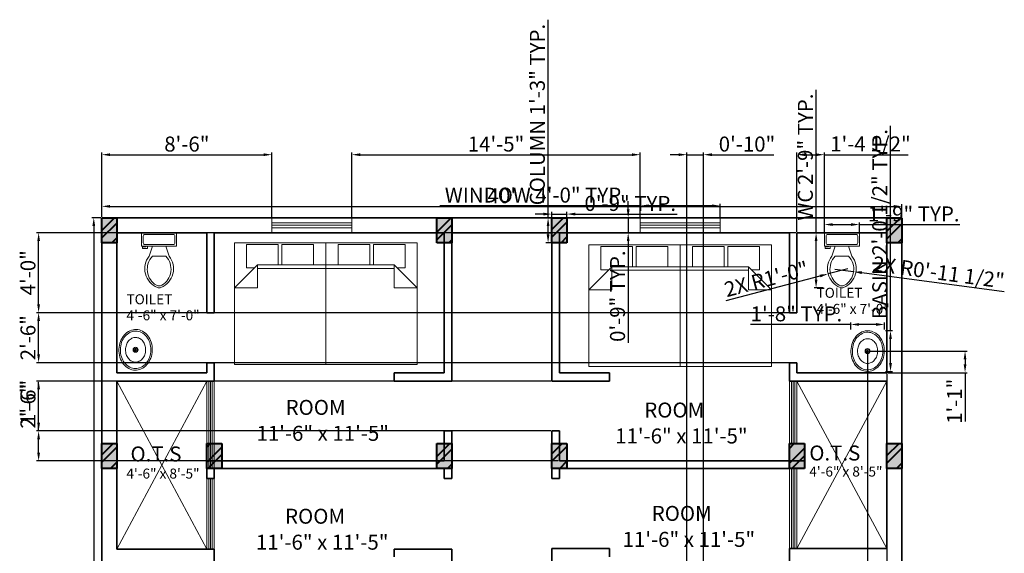
# Model space of a CAD drawing. Units: inches. Extents: x 2507 to 5802, y 1229 to 3238.
# Tile 2 of 2: x 2507 to 3097, y 1794 to 2114. Entities that reach past the tile are written whole.
import ezdxf

# ---------------------------------------------------------------- set-up
doc = ezdxf.new("R2010")
doc.units = ezdxf.units.IN
for name, color, linetype, lineweight, true_color in [('A-ANNO-DIMS', 244, 'Continuous', 18, 0x991b1e), ('A-AREA-IDEN', 146, 'Continuous', 18, 0x105689), ('A-FLOR-FIXT', 244, 'Continuous', 18, 0x991b1e), ('A-FLOR-OPEN', 244, 'Continuous', 13, 0x991b1e), ('A-FURN', 146, 'Continuous', 18, 0x105689), ('A-GLAZ', 146, 'Continuous', 18, 0x105689)]:
    doc.layers.add(name, color=color, linetype=linetype, lineweight=lineweight, true_color=true_color)
doc.layers.add('A-COLS', color=7, linetype='Continuous', lineweight=40)
doc.layers.add('A-WALL', color=7, linetype='Continuous', lineweight=35)
doc.styles.get("Standard").update_dxf_attribs({"font": 'arial.ttf'})
doc.dimstyles.new('ISO-25', dxfattribs={"dimtxt": 9, "dimasz": 5, "dimexe": 1.25, "dimexo": 0.625, "dimtad": 1, "dimdec": 0, "dimlunit": 3, "dimtxsty": 'Standard', "dimcen": 2.5, "dimadec": 0, "dimazin": 0, "dimtfac": 1, "dimtdec": 0, "dimtmove": 0, "dimatfit": 3, "dimfxl": 1, "dimarcsym": 0})
pattern_1 = [(45, (-3102.79, -1462.177), (-6.735192, 6.735192), []), (45, (-3098.3, -1462.177), (-6.735192, 6.735192), [])]

# ---------------------------------------------------------------- blocks, each defined once
blk = doc.blocks.new('Bed - Queen')
for p, q in [((0, -80.00003), (0, 0)), ((0, 0), (59.99999, 0)), ((59.99999, 0), (59.99999, -80.00003)), ((7.99999, -1.2), (28.79998, -1.2)), ((7.99999, -14.4), (7.99999, -1.2)), ((28.79998, -1.2), (28.79998, -14.4)), ((31.19999, -1.2), (51.99999, -1.2)), ((31.19999, -14.4), (31.19999, -1.2)), ((51.99999, -1.2), (51.99999, -16.4)), ((0, -14.4), (44.8, -14.4)), ((44.8, -16.8), (0, -16.8)), ((59.99999, -29.6), (44.8, -14.4)), ((44.8, -14.4), (44.8, -29.6)), ((51.99999, -16.4), (46.79936, -16.4)), ((44.8, -29.6), (59.99999, -29.6)), ((59.99999, -80.00003), (0, -80.00003))]:
    blk.add_line(p, q)
blk = doc.blocks.new('*D2')
at = {"layer": 'A-ANNO-DIMS', "color": 0, "lineweight": -2, "transparency": 16777216}
for p, q in [((2555.99, 1995.72), (2555.99, 2003.23)), ((3035.99, 1995.72), (3035.99, 2003.23)), ((2560.99, 2001.98), (3030.99, 2001.98))]:
    blk.add_line(p, q, dxfattribs=at)
at = {"layer": 'A-ANNO-DIMS', "color": 0, "transparency": 16777216}
for points in [[(2560.99, 2002.81), (2560.99, 2001.15), (2555.99, 2001.98)], [(3030.99, 2002.81), (3030.99, 2001.15), (3035.99, 2001.98)]]:
    blk.add_solid(points, dxfattribs=at)
at = {"layer": 'Defpoints', "color": 0, "transparency": 16777216}
for p in [(3035.99, 2001.98), (2555.99, 1995.09), (3035.99, 1995.09)]:
    blk.add_point(p, dxfattribs=at)
at = {"layer": 'A-ANNO-DIMS', "color": 0, "transparency": 16777216, "insert": (2795.99, 2007.2), "char_height": 9, "attachment_point": 5}
blk.add_mtext("40'", dxfattribs=at)
blk = doc.blocks.new('*D3')
at = {"layer": 'A-ANNO-DIMS', "color": 0, "lineweight": -2, "transparency": 16777216}
for p, q in [((2555.37, 1995.09), (2549.93, 1995.09)), ((2551.18, 1990.09), (2551.18, 1280.09)), ((2555.37, 1275.09), (2549.93, 1275.09))]:
    blk.add_line(p, q, dxfattribs=at)
at = {"layer": 'A-ANNO-DIMS', "color": 0, "transparency": 16777216}
for points in [[(2550.35, 1990.09), (2552.02, 1990.09), (2551.18, 1995.09)], [(2550.35, 1280.09), (2552.02, 1280.09), (2551.18, 1275.09)]]:
    blk.add_solid(points, dxfattribs=at)
at = {"layer": 'Defpoints', "color": 0, "transparency": 16777216}
for p in [(2555.99, 1995.09), (2551.18, 1275.09), (2555.99, 1275.09)]:
    blk.add_point(p, dxfattribs=at)
at = {"layer": 'A-ANNO-DIMS', "color": 0, "transparency": 16777216, "insert": (2545.96, 1635.09), "char_height": 9, "attachment_point": 5, "rotation": 90}
blk.add_mtext("60'", dxfattribs=at)
blk = doc.blocks.new('Toilet - top')
for p, q in [((9.5, -6), (9.5, -2)), ((-10, -8.5), (-8, -8.5)), ((-10, -9.5), (-10, -8.5)), ((-7, -9.5), (-10, -9.5)), ((-8, -8.5), (-8, -8)), ((-7, -8), (-7, -9.5)), ((-4, -8), (-6, -14)), ((4, -8), (6, -14)), ((4, -14), (-4, -14))]:
    blk.add_line(p, q)
blk.add_lwpolyline([(10.5, -8), (10.5, 0), (-10.5, 0), (-10.5, -8)], close=True)
for points in [[(-9.5, -2), (-9.5, -6)], [(8.5, -1), (-8.5, -1)], [(-8.5, -7), (8.5, -7)]]:
    blk.add_lwpolyline(points)
for centre, radius, start, end in [((-8.62, -1.88), 0.884, 81.8699, 188.1301), ((8.62, -1.88), 0.884, 351.8699, 98.1301), ((-8.62, -6.12), 0.884, 171.8699, 278.1301), ((8.62, -6.12), 0.884, 261.8699, 8.1301), ((3.52, -21.58), 12.17, 141.46911, 247.97143), ((4.2, -21.82), 11.33, 136.36773, 238.94682), ((-3.52, -21.58), 12.17, 292.02843, 38.53071), ((-4.2, -21.82), 11.33, 301.05301, 43.63209), ((0, -27.88), 4, 245.73182, 294.26817), ((0, -29), 4, 254.86053, 285.13947)]:
    blk.add_arc(centre, radius, start, end)
blk = doc.blocks.new('Sink - Oval top')
for p, q in [((-1, 0), (1, 0)), ((0, 1), (0, -1))]:
    blk.add_line(p, q)
for points in [[(-12.23, 0.39, 0.117634), (-11.46, -3.36, 0.104469), (-8.88, -6.8, 0.090016), (-5.08, -9.07, 0.08192), (-0.32, -10.02, 0.08192), (4.49, -9.38, 0.090016), (8.42, -7.36, 0.104469), (11.22, -4.09, 0.117634), (12.23, -0.39, 0.117634), (11.46, 3.36, 0.104469), (8.88, 6.8, 0.090016), (5.08, 9.07, 0.08192), (0.32, 10.02, 0.08192), (-4.49, 9.38, 0.090016), (-8.42, 7.36, 0.104469), (-11.22, 4.09, 0.117634)], [(-11.29, 0.16, 0.118622), (-10.52, -3.25, 0.104678), (-8.07, -6.36, 0.089562), (-4.54, -8.37, 0.081185), (-0.13, -9.15, 0.081185), (4.3, -8.49, 0.089562), (7.89, -6.58, 0.104678), (10.42, -3.55, 0.118622), (11.29, -0.16, 0.118622), (10.52, 3.25, 0.104678), (8.07, 6.36, 0.089562), (4.54, 8.37, 0.081185), (0.13, 9.15, 0.081185), (-4.3, 8.49, 0.089562), (-7.89, 6.58, 0.104678), (-10.42, 3.55, 0.118622)], [(-7.42, 0.08, 0.118283), (-6.91, -2.17, 0.104607), (-5.29, -4.21, 0.089718), (-2.97, -5.53, 0.081436), (-0.07, -6.04, 0.081436), (2.84, -5.59, 0.089718), (5.2, -4.33, 0.104607), (6.86, -2.32, 0.118283), (7.42, -0.08, 0.118283), (6.91, 2.17, 0.104607), (5.29, 4.21, 0.089718), (2.97, 5.53, 0.081436), (0.07, 6.04, 0.081436), (-2.84, 5.59, 0.089718), (-5.2, 4.33, 0.104607), (-6.86, 2.32, 0.118283)]]:
    blk.add_lwpolyline(points, format="xyb", close=True)
for radius in [1.5, 1]:
    blk.add_circle((0, 0), radius)
blk = doc.blocks.new('COL-9x15')
h = blk.add_hatch()
h.set_pattern_fill('ANSI32', color=256)
h.set_pattern_definition(pattern_1)
h.paths.add_polyline_path([(9, 15), (0, 15), (0, 0), (9, 0)])
h = blk.add_hatch()
h.set_pattern_fill('ANSI32', color=256)
h.set_pattern_definition(pattern_1)
h.paths.add_polyline_path([(9, 15), (0, 15), (0, 0), (9, 0)])
at = {"transparency": 33554687}
h = blk.add_hatch(dxfattribs=at)
h.set_pattern_fill('ANSI32', color=256)
h.set_pattern_definition(pattern_1)
h.paths.add_polyline_path([(9, 15), (0, 15), (0, 0), (9, 0)])
h = blk.add_hatch(color=256, dxfattribs=at)
h.dxf.hatch_style = 1
h.paths.add_polyline_path([(9, 15), (0, 15), (0, 0), (9, 0)])
for p, q in [((0, 15), (9, 15)), ((0, 0), (0, 15)), ((9, 15), (9, 0)), ((9, 0), (0, 0))]:
    blk.add_line(p, q)
blk = doc.blocks.new('WIN-48x9')
for p, q in [((0, 9), (48, 9)), ((0, 0), (0, 9)), ((0, 6), (48, 6)), ((48, 9), (48, 0)), ((0, 4.5), (48, 4.5)), ((0, 3), (48, 3)), ((48, 0), (0, 0))]:
    blk.add_line(p, q)
blk = doc.blocks.new('*D13')
at = {"layer": 'A-ANNO-DIMS', "color": 0, "lineweight": -2, "transparency": 16777216}
for p, q in [((2823.74, 1995.09), (2823.74, 2114.07)), ((2825.37, 1995.09), (2822.49, 1995.09)), ((2823.74, 1985.09), (2823.74, 1990.09)), ((2825.37, 1980.09), (2822.49, 1980.09))]:
    blk.add_line(p, q, dxfattribs=at)
at = {"layer": 'A-ANNO-DIMS', "color": 0, "transparency": 16777216}
for points in [[(2822.91, 1990.09), (2824.57, 1990.09), (2823.74, 1995.09)], [(2822.91, 1985.09), (2824.57, 1985.09), (2823.74, 1980.09)]]:
    blk.add_solid(points, dxfattribs=at)
at = {"layer": 'Defpoints', "color": 0, "transparency": 16777216}
for p in [(2823.74, 1995.09), (2825.99, 1995.09), (2825.99, 1980.09)]:
    blk.add_point(p, dxfattribs=at)
at = {"layer": 'A-ANNO-DIMS', "color": 0, "transparency": 16777216, "insert": (2818.46, 2057.08), "char_height": 9, "attachment_point": 5, "rotation": 90}
blk.add_mtext('COLUMN 1\'-3" TYP.', dxfattribs=at)
blk = doc.blocks.new('*D14')
at = {"layer": 'A-ANNO-DIMS', "color": 0, "lineweight": -2, "transparency": 16777216}
for p, q in [((2820.99, 1997.34), (2815.99, 1997.34)), ((2825.99, 1995.72), (2825.99, 1998.59)), ((2825.99, 1997.34), (2834.99, 1997.34)), ((2834.99, 1995.72), (2834.99, 1998.59)), ((2839.99, 1997.34), (2901.1, 1997.34))]:
    blk.add_line(p, q, dxfattribs=at)
at = {"layer": 'A-ANNO-DIMS', "color": 0, "transparency": 16777216}
for points in [[(2820.99, 1998.17), (2820.99, 1996.51), (2825.99, 1997.34)], [(2839.99, 1998.17), (2839.99, 1996.51), (2834.99, 1997.34)]]:
    blk.add_solid(points, dxfattribs=at)
at = {"layer": 'Defpoints', "color": 0, "transparency": 16777216}
for p in [(2834.99, 1997.34), (2825.99, 1995.09), (2834.99, 1995.09)]:
    blk.add_point(p, dxfattribs=at)
at = {"layer": 'A-ANNO-DIMS', "color": 0, "transparency": 16777216, "insert": (2873.04, 2002.56), "char_height": 9, "attachment_point": 5}
blk.add_mtext('0\'-9" TYP.', dxfattribs=at)
blk = doc.blocks.new('*D17')
at = {"layer": 'A-ANNO-DIMS', "color": 0, "lineweight": -2, "transparency": 16777216}
for p, q in [((2984.53, 1986.09), (2984.53, 2072.01)), ((2988.87, 1986.09), (2983.28, 1986.09)), ((2984.53, 1958.04), (2984.53, 1981.09)), ((2988.87, 1953.04), (2983.28, 1953.04))]:
    blk.add_line(p, q, dxfattribs=at)
at = {"layer": 'A-ANNO-DIMS', "color": 0, "transparency": 16777216}
for points in [[(2983.7, 1981.09), (2985.37, 1981.09), (2984.53, 1986.09)], [(2983.7, 1958.04), (2985.37, 1958.04), (2984.53, 1953.04)]]:
    blk.add_solid(points, dxfattribs=at)
at = {"layer": 'Defpoints', "color": 0, "transparency": 16777216}
for p in [(2984.53, 1986.09), (2989.49, 1986.09), (2989.49, 1953.04)]:
    blk.add_point(p, dxfattribs=at)
at = {"layer": 'A-ANNO-DIMS', "color": 0, "transparency": 16777216, "insert": (2979.25, 2031.55), "char_height": 9, "attachment_point": 5, "rotation": 90}
blk.add_mtext('WC 2\'-9" TYP.', dxfattribs=at)
blk = doc.blocks.new('*D18')
at = {"layer": 'A-ANNO-DIMS', "color": 0, "lineweight": -2, "transparency": 16777216}
for p, q in [((2989.49, 1986.72), (2989.49, 1992.3)), ((2994.49, 1991.05), (3005.49, 1991.05)), ((3010.49, 1986.72), (3010.49, 1992.3)), ((3010.49, 1991.05), (3070.75, 1991.05))]:
    blk.add_line(p, q, dxfattribs=at)
at = {"layer": 'A-ANNO-DIMS', "color": 0, "transparency": 16777216}
for points in [[(2994.49, 1991.88), (2994.49, 1990.21), (2989.49, 1991.05)], [(3005.49, 1991.88), (3005.49, 1990.21), (3010.49, 1991.05)]]:
    blk.add_solid(points, dxfattribs=at)
at = {"layer": 'Defpoints', "color": 0, "transparency": 16777216}
for p in [(3010.49, 1991.05), (2989.49, 1986.09), (3010.49, 1986.09)]:
    blk.add_point(p, dxfattribs=at)
at = {"layer": 'A-ANNO-DIMS', "color": 0, "transparency": 16777216, "insert": (3043.12, 1996.27), "char_height": 9, "attachment_point": 5}
blk.add_mtext('1\'-9" TYP.', dxfattribs=at)
blk = doc.blocks.new('*D19')
at = {"layer": 'A-ANNO-DIMS', "color": 0, "lineweight": -2, "transparency": 16777216}
for p, q in [((3029.18, 1927.36), (3029.18, 2050.27)), ((3026.12, 1927.36), (3030.43, 1927.36)), ((3029.18, 1907.81), (3029.18, 1922.36)), ((3026.12, 1902.81), (3030.43, 1902.81))]:
    blk.add_line(p, q, dxfattribs=at)
at = {"layer": 'A-ANNO-DIMS', "color": 0, "transparency": 16777216}
for points in [[(3028.34, 1922.36), (3030.01, 1922.36), (3029.18, 1927.36)], [(3028.34, 1907.81), (3030.01, 1907.81), (3029.18, 1902.81)]]:
    blk.add_solid(points, dxfattribs=at)
at = {"layer": 'Defpoints', "color": 0, "transparency": 16777216}
for p in [(3025.49, 1927.36), (3029.18, 1927.36), (3025.49, 1902.81)]:
    blk.add_point(p, dxfattribs=at)
at = {"layer": 'A-ANNO-DIMS', "color": 0, "transparency": 16777216, "insert": (3023.9, 1991.31), "char_height": 9, "attachment_point": 5, "rotation": 90}
blk.add_mtext('BASIN 2\'-0 1/2" TYP.', dxfattribs=at)
blk = doc.blocks.new('*D20')
at = {"layer": 'A-ANNO-DIMS', "color": 0, "lineweight": -2, "transparency": 16777216}
for p, q in [((3005.36, 1927.98), (3005.36, 1932.29)), ((3025.49, 1927.98), (3025.49, 1932.29)), ((3005.36, 1931.04), (2945.1, 1931.04)), ((3020.49, 1931.04), (3010.36, 1931.04))]:
    blk.add_line(p, q, dxfattribs=at)
at = {"layer": 'A-ANNO-DIMS', "color": 0, "transparency": 16777216}
for points in [[(3010.36, 1931.88), (3010.36, 1930.21), (3005.36, 1931.04)], [(3020.49, 1931.88), (3020.49, 1930.21), (3025.49, 1931.04)]]:
    blk.add_solid(points, dxfattribs=at)
at = {"layer": 'Defpoints', "color": 0, "transparency": 16777216}
for p in [(3005.36, 1931.04), (3005.36, 1927.36), (3025.49, 1927.36)]:
    blk.add_point(p, dxfattribs=at)
at = {"layer": 'A-ANNO-DIMS', "color": 0, "transparency": 16777216, "insert": (2972.73, 1936.26), "char_height": 9, "attachment_point": 5}
blk.add_mtext('1\'-8" TYP.', dxfattribs=at)
blk = doc.blocks.new('*D21')
at = {"layer": 'A-ANNO-DIMS', "color": 0, "lineweight": -2, "transparency": 16777216}
for p, q in [((2878.99, 1995.72), (2878.99, 2003.54)), ((2926.99, 1995.72), (2926.99, 2003.54)), ((2878.99, 2002.29), (2758.86, 2002.29)), ((2921.99, 2002.29), (2883.99, 2002.29))]:
    blk.add_line(p, q, dxfattribs=at)
at = {"layer": 'A-ANNO-DIMS', "color": 0, "transparency": 16777216}
for points in [[(2883.99, 2003.12), (2883.99, 2001.46), (2878.99, 2002.29)], [(2921.99, 2003.12), (2921.99, 2001.46), (2926.99, 2002.29)]]:
    blk.add_solid(points, dxfattribs=at)
at = {"layer": 'Defpoints', "color": 0, "transparency": 16777216}
for p in [(2878.99, 2002.29), (2878.99, 1995.09), (2926.99, 1995.09)]:
    blk.add_point(p, dxfattribs=at)
at = {"layer": 'A-ANNO-DIMS', "color": 0, "transparency": 16777216, "insert": (2816.42, 2007.57), "char_height": 9, "attachment_point": 5}
blk.add_mtext('WINDOW 4\'-0" TYP.', dxfattribs=at)
blk = doc.blocks.new('*D22')
at = {"layer": 'A-ANNO-DIMS', "color": 0, "lineweight": -2, "transparency": 16777216}
for p, q in [((2871.79, 2000.09), (2871.79, 2005.09)), ((2878.37, 1995.09), (2870.54, 1995.09)), ((2871.79, 1995.09), (2871.79, 1986.09)), ((2878.37, 1986.09), (2870.54, 1986.09)), ((2871.79, 1981.09), (2871.79, 1919.98))]:
    blk.add_line(p, q, dxfattribs=at)
at = {"layer": 'A-ANNO-DIMS', "color": 0, "transparency": 16777216}
for points in [[(2870.96, 2000.09), (2872.63, 2000.09), (2871.79, 1995.09)], [(2870.96, 1981.09), (2872.63, 1981.09), (2871.79, 1986.09)]]:
    blk.add_solid(points, dxfattribs=at)
at = {"layer": 'Defpoints', "color": 0, "transparency": 16777216}
for p in [(2878.99, 1995.09), (2871.79, 1986.09), (2878.99, 1986.09)]:
    blk.add_point(p, dxfattribs=at)
at = {"layer": 'A-ANNO-DIMS', "color": 0, "transparency": 16777216, "insert": (2866.57, 1948.04), "char_height": 9, "attachment_point": 5, "rotation": 90}
blk.add_mtext('0\'-9" TYP.', dxfattribs=at)
blk = doc.blocks.new('*D25')
at = {"layer": 'A-ANNO-DIMS', "color": 0, "lineweight": -2, "transparency": 16777216}
for p, q in [((2555.99, 1995.72), (2555.99, 2034.24)), ((2560.99, 2032.99), (2653.02, 2032.99)), ((2658.02, 1995.72), (2658.02, 2034.24))]:
    blk.add_line(p, q, dxfattribs=at)
at = {"layer": 'A-ANNO-DIMS', "color": 0, "transparency": 16777216}
for points in [[(2560.99, 2033.82), (2560.99, 2032.16), (2555.99, 2032.99)], [(2653.02, 2033.82), (2653.02, 2032.16), (2658.02, 2032.99)]]:
    blk.add_solid(points, dxfattribs=at)
at = {"layer": 'Defpoints', "color": 0, "transparency": 16777216}
for p in [(2658.02, 2032.99), (2555.99, 1995.09), (2658.02, 1995.09)]:
    blk.add_point(p, dxfattribs=at)
at = {"layer": 'A-ANNO-DIMS', "color": 0, "transparency": 16777216, "insert": (2607.01, 2038.21), "char_height": 9, "attachment_point": 5}
blk.add_mtext('8\'-6"', dxfattribs=at)
blk = doc.blocks.new('*D26')
at = {"layer": 'A-ANNO-DIMS', "color": 0, "lineweight": -2, "transparency": 16777216}
for p, q in [((2706.02, 1995.72), (2706.02, 2034.24)), ((2711.02, 2032.99), (2873.99, 2032.99)), ((2878.99, 1995.72), (2878.99, 2034.24))]:
    blk.add_line(p, q, dxfattribs=at)
at = {"layer": 'A-ANNO-DIMS', "color": 0, "transparency": 16777216}
for points in [[(2711.02, 2033.82), (2711.02, 2032.16), (2706.02, 2032.99)], [(2873.99, 2033.82), (2873.99, 2032.16), (2878.99, 2032.99)]]:
    blk.add_solid(points, dxfattribs=at)
at = {"layer": 'Defpoints', "color": 0, "transparency": 16777216}
for p in [(2878.99, 2032.99), (2706.02, 1995.09), (2878.99, 1995.09)]:
    blk.add_point(p, dxfattribs=at)
at = {"layer": 'A-ANNO-DIMS', "color": 0, "transparency": 16777216, "insert": (2792.51, 2038.21), "char_height": 9, "attachment_point": 5}
blk.add_mtext('14\'-5"', dxfattribs=at)
blk = doc.blocks.new('*D30')
at = {"layer": 'A-ANNO-DIMS', "color": 0, "lineweight": -2, "transparency": 16777216}
for p, q in [((2825.37, 1897.09), (2516.84, 1897.09)), ((2518.09, 1872.09), (2518.09, 1892.09)), ((2825.37, 1867.09), (2516.84, 1867.09))]:
    blk.add_line(p, q, dxfattribs=at)
at = {"layer": 'A-ANNO-DIMS', "color": 0, "transparency": 16777216}
for points in [[(2517.26, 1892.09), (2518.92, 1892.09), (2518.09, 1897.09)], [(2517.26, 1872.09), (2518.92, 1872.09), (2518.09, 1867.09)]]:
    blk.add_solid(points, dxfattribs=at)
at = {"layer": 'Defpoints', "color": 0, "transparency": 16777216}
for p in [(2518.09, 1897.09), (2825.99, 1897.09), (2825.99, 1867.09)]:
    blk.add_point(p, dxfattribs=at)
at = {"layer": 'A-ANNO-DIMS', "color": 0, "transparency": 16777216, "insert": (2512.87, 1882.09), "char_height": 9, "attachment_point": 5, "rotation": 90}
blk.add_mtext('2\'-6"', dxfattribs=at)
blk = doc.blocks.new('*D31')
at = {"layer": 'A-ANNO-DIMS', "color": 0, "lineweight": -2, "transparency": 16777216}
for p, q in [((2518.09, 1867.09), (2518.09, 1896.42)), ((2825.37, 1867.09), (2516.84, 1867.09)), ((2518.09, 1854.09), (2518.09, 1862.09)), ((2829.87, 1849.09), (2516.84, 1849.09))]:
    blk.add_line(p, q, dxfattribs=at)
at = {"layer": 'A-ANNO-DIMS', "color": 0, "transparency": 16777216}
for points in [[(2517.26, 1862.09), (2518.92, 1862.09), (2518.09, 1867.09)], [(2517.26, 1854.09), (2518.92, 1854.09), (2518.09, 1849.09)]]:
    blk.add_solid(points, dxfattribs=at)
at = {"layer": 'Defpoints', "color": 0, "transparency": 16777216}
for p in [(2518.09, 1867.09), (2825.99, 1867.09), (2830.49, 1849.09)]:
    blk.add_point(p, dxfattribs=at)
at = {"layer": 'A-ANNO-DIMS', "color": 0, "transparency": 16777216, "insert": (2512.87, 1884.25), "char_height": 9, "attachment_point": 5, "rotation": 90}
blk.add_mtext('1\'-6"', dxfattribs=at)
blk = doc.blocks.new('*D32')
at = {"layer": 'A-ANNO-DIMS', "color": 0, "lineweight": -2, "transparency": 16777216}
for p, q in [((2972.37, 1938.09), (2516.84, 1938.09)), ((2518.09, 1913.09), (2518.09, 1933.09)), ((2972.37, 1908.09), (2516.84, 1908.09))]:
    blk.add_line(p, q, dxfattribs=at)
at = {"layer": 'A-ANNO-DIMS', "color": 0, "transparency": 16777216}
for points in [[(2517.26, 1933.09), (2518.92, 1933.09), (2518.09, 1938.09)], [(2517.26, 1913.09), (2518.92, 1913.09), (2518.09, 1908.09)]]:
    blk.add_solid(points, dxfattribs=at)
at = {"layer": 'Defpoints', "color": 0, "transparency": 16777216}
for p in [(2518.09, 1938.09), (2972.99, 1938.09), (2972.99, 1908.09)]:
    blk.add_point(p, dxfattribs=at)
at = {"layer": 'A-ANNO-DIMS', "color": 0, "transparency": 16777216, "insert": (2512.87, 1923.09), "char_height": 9, "attachment_point": 5, "rotation": 90}
blk.add_mtext('2\'-6"', dxfattribs=at)
blk = doc.blocks.new('*D33')
at = {"layer": 'A-ANNO-DIMS', "color": 0, "lineweight": -2, "transparency": 16777216}
for p, q in [((2972.37, 1986.09), (2516.84, 1986.09)), ((2518.09, 1943.09), (2518.09, 1981.09)), ((2972.37, 1938.09), (2516.84, 1938.09))]:
    blk.add_line(p, q, dxfattribs=at)
at = {"layer": 'A-ANNO-DIMS', "color": 0, "transparency": 16777216}
for points in [[(2517.26, 1981.09), (2518.92, 1981.09), (2518.09, 1986.09)], [(2517.26, 1943.09), (2518.92, 1943.09), (2518.09, 1938.09)]]:
    blk.add_solid(points, dxfattribs=at)
at = {"layer": 'Defpoints', "color": 0, "transparency": 16777216}
for p in [(2518.09, 1986.09), (2972.99, 1986.09), (2972.99, 1938.09)]:
    blk.add_point(p, dxfattribs=at)
at = {"layer": 'A-ANNO-DIMS', "color": 0, "transparency": 16777216, "insert": (2512.87, 1962.09), "char_height": 9, "attachment_point": 5, "rotation": 90}
blk.add_mtext('4\'-0"', dxfattribs=at)
blk = doc.blocks.new('*D34')
at = {"layer": 'A-ANNO-DIMS', "color": 0, "lineweight": -2, "transparency": 16777216}
for p, q in [((2901.99, 2032.99), (2896.99, 2032.99)), ((2906.99, 1344.72), (2906.99, 2034.24)), ((2906.99, 2032.99), (2916.99, 2032.99)), ((2916.99, 1344.72), (2916.99, 2034.24)), ((2921.99, 2032.99), (2959.16, 2032.99))]:
    blk.add_line(p, q, dxfattribs=at)
at = {"layer": 'A-ANNO-DIMS', "color": 0, "transparency": 16777216}
for points in [[(2901.99, 2033.82), (2901.99, 2032.16), (2906.99, 2032.99)], [(2921.99, 2033.82), (2921.99, 2032.16), (2916.99, 2032.99)]]:
    blk.add_solid(points, dxfattribs=at)
at = {"layer": 'Defpoints', "color": 0, "transparency": 16777216}
for p in [(2916.99, 2032.99), (2906.99, 1344.09), (2916.99, 1344.09)]:
    blk.add_point(p, dxfattribs=at)
at = {"layer": 'A-ANNO-DIMS', "color": 0, "transparency": 16777216, "insert": (2943.07, 2038.21), "char_height": 9, "attachment_point": 5}
blk.add_mtext('0\'-10"', dxfattribs=at)
blk = doc.blocks.new('*D36')
at = {"layer": 'A-ANNO-DIMS', "color": 0, "lineweight": -2, "transparency": 16777216}
for p, q in [((2972.99, 1986.72), (2972.99, 2034.24)), ((2977.99, 2032.99), (2984.49, 2032.99)), ((2989.49, 1986.72), (2989.49, 2034.24)), ((2989.49, 2032.99), (3039.79, 2032.99))]:
    blk.add_line(p, q, dxfattribs=at)
at = {"layer": 'A-ANNO-DIMS', "color": 0, "transparency": 16777216}
for points in [[(2977.99, 2033.82), (2977.99, 2032.16), (2972.99, 2032.99)], [(2984.49, 2033.82), (2984.49, 2032.16), (2989.49, 2032.99)]]:
    blk.add_solid(points, dxfattribs=at)
at = {"layer": 'Defpoints', "color": 0, "transparency": 16777216}
for p in [(2989.49, 2032.99), (2972.99, 1986.09), (2989.49, 1986.09)]:
    blk.add_point(p, dxfattribs=at)
at = {"layer": 'A-ANNO-DIMS', "color": 0, "transparency": 16777216, "insert": (3017.14, 2038.27), "char_height": 9, "attachment_point": 5}
blk.add_mtext('1\'-4 1/2"', dxfattribs=at)
blk = doc.blocks.new('*D37')
at = {"layer": 'A-ANNO-DIMS', "color": 0, "lineweight": -2, "transparency": 16777216}
for p, q in [((3015.43, 1914.46), (3015.43, 1235.94)), ((3026.99, 1901.47), (3026.99, 1235.94)), ((3020.43, 1237.19), (3021.99, 1237.19)), ((3026.99, 1237.19), (3085.13, 1237.19))]:
    blk.add_line(p, q, dxfattribs=at)
at = {"layer": 'A-ANNO-DIMS', "color": 0, "transparency": 16777216}
for points in [[(3020.43, 1238.02), (3020.43, 1236.36), (3015.43, 1237.19)], [(3021.99, 1238.02), (3021.99, 1236.36), (3026.99, 1237.19)]]:
    blk.add_solid(points, dxfattribs=at)
at = {"layer": 'Defpoints', "color": 0, "transparency": 16777216}
for p in [(3015.43, 1915.08), (3026.99, 1902.09), (3026.99, 1237.19)]:
    blk.add_point(p, dxfattribs=at)
at = {"layer": 'A-ANNO-DIMS', "color": 0, "transparency": 16777216, "insert": (3058.56, 1242.47), "char_height": 9, "attachment_point": 5}
blk.add_mtext('0\'-11 1/2"', dxfattribs=at)
blk = doc.blocks.new('*D38')
at = {"layer": 'A-ANNO-DIMS', "color": 0, "lineweight": -2, "transparency": 16777216}
for p, q in [((3016.05, 1915.08), (3075.14, 1915.08)), ((3073.89, 1910.08), (3073.89, 1907.09)), ((3027.62, 1902.09), (3075.14, 1902.09)), ((3073.89, 1902.09), (3073.89, 1872.76))]:
    blk.add_line(p, q, dxfattribs=at)
at = {"layer": 'A-ANNO-DIMS', "color": 0, "transparency": 16777216}
for points in [[(3073.06, 1910.08), (3074.72, 1910.08), (3073.89, 1915.08)], [(3073.06, 1907.09), (3074.72, 1907.09), (3073.89, 1902.09)]]:
    blk.add_solid(points, dxfattribs=at)
at = {"layer": 'Defpoints', "color": 0, "transparency": 16777216}
for p in [(3015.43, 1915.08), (3026.99, 1902.09), (3073.89, 1902.09)]:
    blk.add_point(p, dxfattribs=at)
at = {"layer": 'A-ANNO-DIMS', "color": 0, "transparency": 16777216, "insert": (3068.75, 1884.93), "char_height": 9, "attachment_point": 5, "rotation": 90}
blk.add_mtext('1\'-1"', dxfattribs=at)
blk = doc.blocks.new('*D39')
at = {"layer": 'A-ANNO-DIMS', "color": 0, "lineweight": -2, "transparency": 16777216}
for p, q in [((3003.51, 1964.51), (2991.74, 1961.42)), ((2930.54, 1945.34), (2986.9, 1960.15))]:
    blk.add_line(p, q, dxfattribs=at)
at = {"layer": 'A-ANNO-DIMS', "color": 0, "transparency": 16777216}
blk.add_solid([(2986.69, 1960.95), (2987.12, 1959.34), (2991.74, 1961.42)], dxfattribs=at)
at = {"layer": 'Defpoints', "color": 0, "transparency": 16777216}
for p in [(2991.74, 1961.42), (3003.51, 1964.51)]:
    blk.add_point(p, dxfattribs=at)
at = {"layer": 'A-ANNO-DIMS', "color": 0, "transparency": 16777216, "insert": (2954.98, 1957.16), "char_height": 9, "attachment_point": 5, "rotation": 14.72153}
blk.add_mtext('2X R1\'-0"', dxfattribs=at)
blk = doc.blocks.new('*D40')
at = {"layer": 'A-ANNO-DIMS', "color": 0, "lineweight": -2, "transparency": 16777216}
for p, q in [((2995.79, 1964.27), (3007.02, 1962.76)), ((3097.45, 1950.61), (3011.97, 1962.1))]:
    blk.add_line(p, q, dxfattribs=at)
at = {"layer": 'A-ANNO-DIMS', "color": 0, "transparency": 16777216}
blk.add_solid([(3012.08, 1962.92), (3011.86, 1961.27), (3007.02, 1962.76)], dxfattribs=at)
at = {"layer": 'Defpoints', "color": 0, "transparency": 16777216}
for p in [(2995.79, 1964.27), (3007.02, 1962.76)]:
    blk.add_point(p, dxfattribs=at)
at = {"layer": 'A-ANNO-DIMS', "color": 0, "transparency": 16777216, "insert": (3057.89, 1961.25), "char_height": 9, "attachment_point": 5, "rotation": 352.34378}
blk.add_mtext('2X R0\'-11 1/2"', dxfattribs=at)

msp = doc.modelspace()

# ---------------------------------------------------------------- linework, layer by layer
at = {"layer": 'A-FLOR-OPEN'}
for p, q in [((2564.99, 1897.09), (2618.99, 1796.09)), ((2564.99, 1796.09), (2618.99, 1897.09)), ((2972.99, 1897.09), (3026.99, 1796.59)), ((2972.99, 1796.59), (3026.99, 1897.09))]:
    msp.add_line(p, q, dxfattribs=at)
at = {"layer": 'A-GLAZ'}
for p, q in [((2618.99, 1897.09), (2618.99, 1844.59)), ((2618.99, 1897.09), (2623.49, 1897.09)), ((2620.24, 1897.09), (2620.24, 1844.59)), ((2621.24, 1897.09), (2621.24, 1844.59)), ((2622.24, 1897.09), (2622.24, 1844.59)), ((2623.49, 1897.09), (2623.49, 1844.59)), ((2968.49, 1897.09), (2972.99, 1897.09)), ((2968.49, 1897.09), (2968.49, 1859.59)), ((2969.74, 1897.09), (2969.74, 1859.59)), ((2970.74, 1897.09), (2970.74, 1859.59)), ((2971.74, 1897.09), (2971.74, 1859.59)), ((2972.99, 1897.09), (2972.99, 1859.59)), ((2968.49, 1796.59), (2968.49, 1844.59)), ((2969.74, 1796.59), (2969.74, 1844.59)), ((2970.74, 1796.59), (2970.74, 1844.59)), ((2971.74, 1796.59), (2971.74, 1844.59)), ((2972.99, 1796.59), (2972.99, 1844.59)), ((2618.99, 1838.59), (2618.99, 1796.09)), ((2620.24, 1838.59), (2620.24, 1796.09)), ((2621.24, 1838.59), (2621.24, 1796.09)), ((2622.24, 1838.59), (2622.24, 1796.09)), ((2623.49, 1838.59), (2623.49, 1796.09)), ((2968.49, 1796.59), (2972.99, 1796.59))]:
    msp.add_line(p, q, dxfattribs=at)
at = {"layer": 'A-WALL'}
for p, q in [((2555.99, 1995.09), (3035.99, 1995.09)), ((2555.99, 1275.09), (2555.99, 1995.09)), ((3035.99, 1995.09), (3035.99, 1275.09)), ((2564.99, 1986.09), (2618.99, 1986.09)), ((2564.99, 1902.09), (2564.99, 1986.09)), ((2618.99, 1938.09), (2618.99, 1986.09)), ((2623.49, 1938.09), (2623.49, 1986.09)), ((2623.49, 1986.09), (2761.49, 1986.09)), ((2761.49, 1902.09), (2761.49, 1986.09)), ((2765.99, 1897.09), (2765.99, 1986.09)), ((2765.99, 1986.09), (2825.99, 1986.09)), ((2825.99, 1908.09), (2825.99, 1986.09)), ((2830.49, 1908.09), (2830.49, 1986.09)), ((2830.49, 1986.09), (2968.49, 1986.09)), ((2968.49, 1938.09), (2968.49, 1986.09)), ((2972.99, 1938.09), (2972.99, 1986.09)), ((2972.99, 1986.09), (3026.99, 1986.09)), ((3026.99, 1986.09), (3026.99, 1902.09)), ((2618.99, 1938.09), (2623.49, 1938.09)), ((2968.49, 1938.09), (2972.99, 1938.09)), ((2618.99, 1902.09), (2618.99, 1908.09)), ((2618.99, 1908.09), (2623.49, 1908.09)), ((2618.99, 1908.09), (2623.49, 1908.09)), ((2623.49, 1897.09), (2623.49, 1908.09)), ((2825.99, 1897.09), (2825.99, 1908.09)), ((2830.49, 1902.09), (2830.49, 1908.09)), ((2968.49, 1908.09), (2972.99, 1908.09)), ((2968.49, 1897.09), (2968.49, 1908.09)), ((2972.99, 1902.09), (2972.99, 1908.09)), ((2564.99, 1902.09), (2618.99, 1902.09)), ((2564.99, 1902.09), (2618.99, 1902.09)), ((2731.49, 1897.09), (2731.49, 1902.09)), ((2731.49, 1902.09), (2761.49, 1902.09)), ((2731.49, 1902.09), (2761.49, 1902.09)), ((2830.49, 1902.09), (2860.49, 1902.09)), ((2860.49, 1897.09), (2860.49, 1902.09)), ((2972.99, 1902.09), (3026.99, 1902.09)), ((2564.99, 1897.09), (2623.49, 1897.09)), ((2564.99, 1897.09), (2623.49, 1897.09)), ((2564.99, 1796.09), (2564.99, 1897.09)), ((2731.49, 1897.09), (2765.99, 1897.09)), ((2731.49, 1897.09), (2765.99, 1897.09)), ((2825.99, 1897.09), (2860.49, 1897.09)), ((2968.49, 1897.09), (3026.99, 1897.09)), ((3026.99, 1897.09), (3026.99, 1849.09)), ((2761.49, 1867.09), (2765.99, 1867.09)), ((2761.49, 1849.09), (2761.49, 1867.09)), ((2765.99, 1838.59), (2765.99, 1867.09)), ((2825.99, 1867.09), (2830.49, 1867.09)), ((2825.99, 1838.59), (2825.99, 1867.09)), ((2830.49, 1849.09), (2830.49, 1867.09)), ((2618.99, 1849.09), (2761.49, 1849.09)), ((2618.99, 1844.59), (2618.99, 1849.09)), ((2830.49, 1849.09), (2977.49, 1849.09)), ((2618.99, 1838.59), (2618.99, 1844.59)), ((2623.49, 1844.59), (2761.49, 1844.59)), ((2623.49, 1838.59), (2623.49, 1844.59)), ((2761.49, 1838.59), (2761.49, 1844.59)), ((2830.49, 1844.59), (2977.49, 1844.59)), ((2830.49, 1838.59), (2830.49, 1844.59)), ((3026.99, 1844.59), (3026.99, 1796.59)), ((2618.99, 1838.59), (2623.49, 1838.59)), ((2761.49, 1838.59), (2765.99, 1838.59)), ((2825.99, 1838.59), (2830.49, 1838.59)), ((2564.99, 1796.09), (2623.49, 1796.09)), ((2623.49, 1785.59), (2623.49, 1796.09)), ((2731.49, 1791.59), (2731.49, 1796.09)), ((2731.49, 1796.09), (2765.99, 1796.09)), ((2765.99, 1755.59), (2765.99, 1796.09)), ((2825.99, 1755.59), (2825.99, 1796.59)), ((2825.99, 1796.59), (2860.49, 1796.59)), ((2860.49, 1791.59), (2860.49, 1796.59)), ((2968.49, 1796.59), (2972.99, 1796.59)), ((2968.49, 1785.59), (2968.49, 1796.59)), ((2968.49, 1796.59), (3026.99, 1796.59))]:
    msp.add_line(p, q, dxfattribs=at)

# ---------------------------------------------------------------- block references
at = {"layer": 'A-COLS'}
for p in [(2555.99, 1980.09), (2756.99, 1980.09), (2825.99, 1980.09), (3026.99, 1980.09), (2555.99, 1844.59), (2618.99, 1844.59), (2756.99, 1844.59), (2825.99, 1844.59), (2968.49, 1844.59), (3026.99, 1844.59)]:
    msp.add_blockref('COL-9x15', p, dxfattribs=at)
at = {"layer": 'A-FLOR-FIXT'}
for p in [(2590.4, 1986.09), (2999.99, 1986.09)]:
    msp.add_blockref('Toilet - top', p, dxfattribs=at)
at = {"layer": 'A-FLOR-FIXT', "rotation": 90}
for p in [(2576.27, 1915.83), (3015.43, 1915.08)]:
    msp.add_blockref('Sink - Oval top', p, dxfattribs=at)
at = {"layer": 'A-FURN', "yscale": 0.9146343891503859, "zscale": 0.9146343891503859}
for p, xscale in [((2690.4, 1980.09), -0.9146343891503859), ((2690.4, 1980.09), 0.9146343891503859), ((2902.99, 1978.92), -0.9146343891503859), ((2902.99, 1978.92), 0.9146343891503859)]:
    msp.add_blockref('Bed - Queen', p, dxfattribs=dict(at, xscale=xscale))
at = {"layer": 'A-GLAZ', "rotation": 180}
for p in [(2706.02, 1995.09), (2926.99, 1995.09)]:
    msp.add_blockref('WIN-48x9', p, dxfattribs=at)

# ---------------------------------------------------------------- texts
at = {"layer": 'A-AREA-IDEN'}
for s, height, p in [('TOILET', 6, (2984.8, 1947.06)), ('TOILET', 6, (2570.81, 1943.17)), ('4\'-6" x 7\'-0"', 6, (2984.8, 1937.42)), ('4\'-6" x 7\'-0"', 6, (2570.81, 1933.53)), ('ROOM', 9, (2666.26, 1876.75)), ('ROOM', 9, (2881.44, 1875.16)), ('11\'-6" x 11\'-5"', 9, (2648.8, 1861.17)), ('11\'-6" x 11\'-5"', 9, (2863.97, 1859.58)), ('O.T.S', 9, (2573.2, 1848.78)), ('O.T.S', 9, (2980.45, 1849.36)), ('4\'-6" x 8\'-5"', 6, (2570.74, 1838.51)), ('4\'-6" x 8\'-5"', 6, (2980.45, 1839.72)), ('ROOM', 9, (2665.95, 1811.38)), ('ROOM', 9, (2885.92, 1813.08)), ('11\'-6" x 11\'-5"', 9, (2648.49, 1795.8)), ('11\'-6" x 11\'-5"', 9, (2868.45, 1797.5))]:
    msp.add_text(s, height=height, dxfattribs=at).set_placement(p)

# ---------------------------------------------------------------- dimensions: what is measured, and where the dimension line sits
at = {"layer": 'A-ANNO-DIMS'}
for base, p1, p2, angle, text, picture, middle in [((2823.74, 1995.09), (2825.99, 1980.09), (2825.99, 1995.09), 90, 'COLUMN <> TYP.', '*D13', (2818.46, 2057.08)), ((2984.5333, 1986.091), (2989.4902, 1953.0447), (2989.4902, 1986.091), 90, 'WC <> TYP.', '*D17', (2979.2548, 2031.5499)), ((3029.1776, 1927.3595), (3025.495, 1902.8086), (3025.495, 1927.3595), 90, 'BASIN <> TYP.', '*D19', (3023.8991, 1991.3126)), ((2878.99, 2002.29), (2926.99, 1995.09), (2878.99, 1995.09), 180, 'WINDOW <> TYP.', '*D21', (2816.42, 2007.57)), ((2871.79, 1986.09), (2878.99, 1995.09), (2878.99, 1986.09), 270, '<> TYP.', '*D22', (2866.57, 1948.04)), ((3005.36, 1931.04), (3025.49, 1927.36), (3005.36, 1927.36), 180, '<> TYP.', '*D20', (2972.73, 1936.26))]:
    dim = msp.add_linear_dim(base=base, p1=p1, p2=p2, angle=angle, text=text, dimstyle='ISO-25', override={"dimdec": 1, "dimlfac": 1, "dimrnd": 0, "dimzin": 1, "dimdsep": 46, "dimlunit": 4, "dimfrac": 2}, dxfattribs=at)
    dim.commit()
    dim.dimension.update_dxf_attribs({"geometry": picture, "text_midpoint": middle})
for base, p1, p2, override, picture, middle in [((2989.49, 2032.99), (2972.99, 1986.09), (2989.49, 1986.09), {"dimdec": 1, "dimlfac": 1, "dimrnd": 0, "dimzin": 1, "dimdsep": 46, "dimlunit": 4, "dimfrac": 2}, '*D36', (3017.14, 2038.27)), ((2658.02, 2032.99), (2555.99, 1995.09), (2658.02, 1995.09), {"dimdec": 1, "dimlfac": 1, "dimrnd": 0, "dimzin": 1, "dimdsep": 46, "dimlunit": 4, "dimfrac": 2}, '*D25', (2607.01, 2038.21)), ((2878.99, 2032.99), (2706.02, 1995.09), (2878.99, 1995.09), {"dimdec": 1, "dimlfac": 1, "dimrnd": 0, "dimzin": 1, "dimdsep": 46, "dimlunit": 4, "dimfrac": 2}, '*D26', (2792.51, 2038.21)), ((2916.99, 2032.99), (2906.99, 1344.09), (2916.99, 1344.09), {"dimdec": 1, "dimlfac": 1, "dimrnd": 0, "dimzin": 1, "dimdsep": 46, "dimlunit": 4, "dimfrac": 2}, '*D34', (2943.07, 2038.21)), ((3035.99, 2001.98), (2555.99, 1995.09), (3035.99, 1995.09), {"dimclrd": 0, "dimclre": 0, "dimclrt": 0}, '*D2', (2795.99, 2007.2)), ((3026.99, 1237.19), (3015.43, 1915.08), (3026.99, 1902.09), {"dimdec": 1, "dimlfac": 1, "dimrnd": 0, "dimzin": 1, "dimdsep": 46, "dimlunit": 4, "dimfrac": 2}, '*D37', (3058.56, 1242.47))]:
    dim = msp.add_linear_dim(base=base, p1=p1, p2=p2, dimstyle='ISO-25', override=override, dxfattribs=at)
    dim.commit()
    dim.dimension.update_dxf_attribs({"geometry": picture, "text_midpoint": middle})
for base, p1, p2, picture, middle in [((2834.99, 1997.34), (2825.99, 1995.09), (2834.99, 1995.09), '*D14', (2873.04, 2002.56)), ((3010.49, 1991.05), (2989.49, 1986.09), (3010.49, 1986.09), '*D18', (3043.12, 1996.27))]:
    dim = msp.add_linear_dim(base=base, p1=p1, p2=p2, text='<> TYP.', dimstyle='ISO-25', override={"dimdec": 1, "dimlfac": 1, "dimrnd": 0, "dimzin": 1, "dimdsep": 46, "dimlunit": 4, "dimfrac": 2}, dxfattribs=at)
    dim.commit()
    dim.dimension.update_dxf_attribs({"geometry": picture, "text_midpoint": middle})
for base, p1, p2, override, picture, middle in [((2551.18, 1275.09), (2555.99, 1995.09), (2555.99, 1275.09), {"dimclrd": 0, "dimclre": 0, "dimclrt": 0}, '*D3', (2545.96, 1635.09)), ((2518.09, 1986.09), (2972.99, 1938.09), (2972.99, 1986.09), {"dimdec": 1, "dimlfac": 1, "dimrnd": 0, "dimzin": 1, "dimdsep": 46, "dimlunit": 4, "dimfrac": 2}, '*D33', (2512.87, 1962.09)), ((2518.09, 1938.09), (2972.99, 1908.09), (2972.99, 1938.09), {"dimdec": 1, "dimlfac": 1, "dimrnd": 0, "dimzin": 1, "dimdsep": 46, "dimlunit": 4, "dimfrac": 2}, '*D32', (2512.87, 1923.09)), ((3073.89, 1902.09), (3015.43, 1915.08), (3026.99, 1902.09), {"dimdec": 1, "dimlfac": 1, "dimrnd": 0, "dimzin": 1, "dimdsep": 46, "dimlunit": 4, "dimfrac": 2}, '*D38', (3068.75, 1884.93)), ((2518.09, 1867.09), (2830.49, 1849.09), (2825.99, 1867.09), {"dimdec": 1, "dimlfac": 1, "dimrnd": 0, "dimzin": 1, "dimdsep": 46, "dimlunit": 4, "dimfrac": 2}, '*D31', (2512.87, 1884.25)), ((2518.09, 1897.09), (2825.99, 1867.09), (2825.99, 1897.09), {"dimdec": 1, "dimlfac": 1, "dimrnd": 0, "dimzin": 1, "dimdsep": 46, "dimlunit": 4, "dimfrac": 2}, '*D30', (2512.87, 1882.09))]:
    dim = msp.add_linear_dim(base=base, p1=p1, p2=p2, angle=90, dimstyle='ISO-25', override=override, dxfattribs=at)
    dim.commit()
    dim.dimension.update_dxf_attribs({"geometry": picture, "text_midpoint": middle})
for center, mpoint, picture, middle in [((2995.79, 1964.27), (3007.02, 1962.76), '*D40', (3057.89, 1961.25)), ((3003.51, 1964.51), (2991.74, 1961.42), '*D39', (2954.98, 1957.16))]:
    dim = msp.add_radius_dim(center=center, mpoint=mpoint, text='2X <>', dimstyle='ISO-25', override={"dimdec": 1, "dimlfac": 1, "dimrnd": 0, "dimzin": 1, "dimdsep": 46, "dimlunit": 4, "dimfrac": 2}, dxfattribs=at)
    dim.commit()
    dim.dimension.update_dxf_attribs({"geometry": picture, "text_midpoint": middle})

doc.saveas('drawing.dxf')
